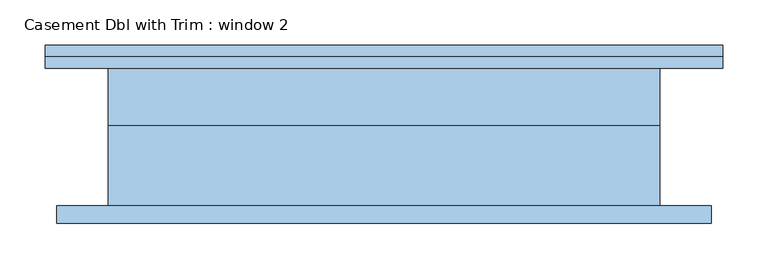
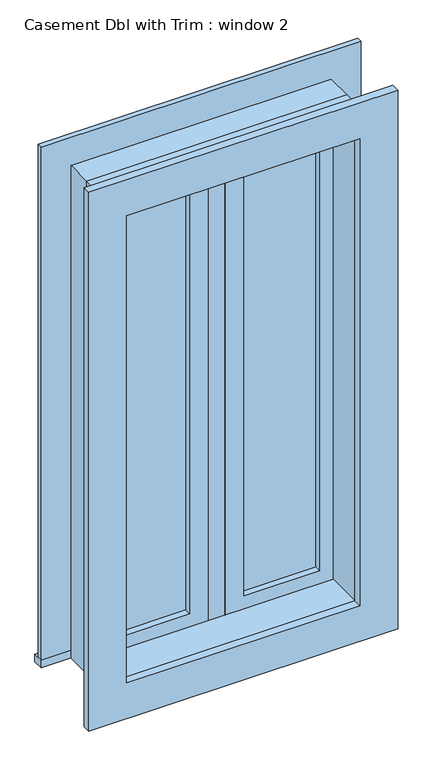
"""IFC4 building model written with IfcOpenShell, lengths in millimetres: window geometry, Casement Dbl with Trim : window 2."""

from ifc_helpers import new_model, si_unit, frame, origin, place, context, project, spatial, polyline, outline, extrude, source, transform, mapped, element, save


def casement_dbl_with_trim_window_2_b083d55d(model_context):
    return source(origin(), model_context, "Body", "SweptSolid", [
        extrude(outline(polyline([(63.5, 60.325), (241.3, 60.325), (241.3, 47.625), (63.5, 47.625), (63.5, 60.325)])), frame((0.0, 0.0, 977.9), z_axis=(0.0, 0.0, 1.0), x_axis=(1.0, 0.0, 0.0)), (0.0, 0.0, 1.0), 1092.2),
        extrude(outline(polyline([(2114.55, 19.05), (933.45, 19.05), (933.45, 285.75), (2114.55, 285.75), (2114.55, 19.05)]), holes=[polyline([(2070.1, 63.5), (2070.1, 241.3), (977.9, 241.3), (977.9, 63.5), (2070.1, 63.5)])]), frame((0.0, 31.75, 0.0), z_axis=(0.0, 1.0, 0.0), x_axis=(0.0, 0.0, 1.0)), (0.0, 0.0, 1.0), 44.45),
        extrude(outline(polyline([(19.05, 31.75), (-19.05, 31.75), (-19.05, 95.25), (19.05, 95.25), (19.05, 31.75)])), frame((0.0, 0.0, 933.45), z_axis=(0.0, 0.0, 1.0), x_axis=(1.0, 0.0, 0.0)), (0.0, 0.0, 1.0), 1181.1),
        extrude(outline(polyline([(-374.65, 120.65), (374.65, 120.65), (374.65, 95.25), (-374.65, 95.25), (-374.65, 120.65)])), frame((0.0, 0.0, 914.4), z_axis=(0.0, 0.0, 1.0), x_axis=(1.0, 0.0, 0.0)), (0.0, 0.0, 1.0), 19.05),
        extrude(outline(polyline([(2114.55, -285.75), (2114.55, 285.75), (933.45, 285.75), (933.45, 374.65), (2203.45, 374.65), (2203.45, -374.65), (933.45, -374.65), (933.45, -285.75), (2114.55, -285.75)])), frame((0.0, 95.25, 0.0), z_axis=(0.0, 1.0, 0.0), x_axis=(0.0, 0.0, 1.0)), (0.0, 0.0, 1.0), 12.7),
        extrude(outline(polyline([(2190.75, 361.95), (2190.75, -361.95), (857.25, -361.95), (857.25, 361.95), (2190.75, 361.95)]), holes=[polyline([(2101.85, 273.05), (946.15, 273.05), (946.15, -273.05), (2101.85, -273.05), (2101.85, 273.05)])]), frame((0.0, -76.2, 0.0), z_axis=(0.0, 1.0, 0.0), x_axis=(0.0, 0.0, 1.0)), (0.0, 0.0, 1.0), 19.05),
        extrude(outline(polyline([(-63.5, 47.625), (-241.3, 47.625), (-241.3, 60.325), (-63.5, 60.325), (-63.5, 47.625)])), frame((0.0, 0.0, 977.9), z_axis=(0.0, 0.0, 1.0), x_axis=(1.0, 0.0, 0.0)), (0.0, 0.0, 1.0), 1092.2),
        extrude(outline(polyline([(2114.55, -285.75), (933.45, -285.75), (933.45, -19.05), (2114.55, -19.05), (2114.55, -285.75)]), holes=[polyline([(2070.1, -241.3), (2070.1, -63.5), (977.9, -63.5), (977.9, -241.3), (2070.1, -241.3)])]), frame((0.0, 31.75, 0.0), z_axis=(0.0, 1.0, 0.0), x_axis=(0.0, 0.0, 1.0)), (0.0, 0.0, 1.0), 44.45),
        extrude(outline(polyline([(2133.6, -304.8), (914.4, -304.8), (914.4, 304.8), (2133.6, 304.8), (2133.6, -304.8)]), holes=[polyline([(2101.85, -273.05), (2101.85, 273.05), (946.15, 273.05), (946.15, -273.05), (2101.85, -273.05)])]), frame((0.0, -57.15, 0.0), z_axis=(0.0, 1.0, 0.0), x_axis=(0.0, 0.0, 1.0)), (0.0, 0.0, 1.0), 88.9),
        extrude(outline(polyline([(2133.6, 304.8), (2133.6, -304.8), (914.4, -304.8), (914.4, 304.8), (2133.6, 304.8)]), holes=[polyline([(2114.55, 285.75), (933.45, 285.75), (933.45, -285.75), (2114.55, -285.75), (2114.55, 285.75)])]), frame((0.0, 31.75, 0.0), z_axis=(0.0, 1.0, 0.0), x_axis=(0.0, 0.0, 1.0)), (0.0, 0.0, 1.0), 63.5),
    ])


if __name__ == "__main__":
    model = new_model("IFC4")
    model_context = context("Model", 3, world=origin())
    ifc_project = project(units=[si_unit("LENGTHUNIT", "METRE", prefix="MILLI")], contexts=[model_context])
    site = spatial("IfcSite", under=ifc_project)
    building = spatial("IfcBuilding", under=site)
    placement = place(None, origin())
    casement_dbl_with_trim_window_2_shape = casement_dbl_with_trim_window_2_b083d55d(model_context)
    element("IfcWindow", 1, ObjectType="Casement Dbl with Trim : window 2", at=placement, inside=building, context=model_context, shape_type="MappedRepresentation", body=[
        mapped(casement_dbl_with_trim_window_2_shape, transform((0.0, 0.0, 0.0), x_axis=(1.0, 0.0, 0.0), y_axis=(0.0, 1.0, 0.0), z_axis=(0.0, 0.0, 1.0))),
    ])
    save(model, "model.ifc")

# Revit data of these elements
# Type "Casement Dbl with Trim : window 2"
#   Type Mark = "13"
#   Construction Type Id = "GSP4R"
#   Assembly Code = "B2020100"
#   Analytic Construction = "1/8 in Pilkington single glazing"
#   Visual Light Transmittance = 0.9
#   Solar Heat Gain Coefficient = 0.78
#   Heat Transfer Coefficient (U) = 0.6496 BTU/(h·ft²·°F)
#   Height = 4' - 0"
#   Default Sill Height = 3' - 0"
#   Trim Projection - Ext. = 0' - 0 1/2"
#   Trim Projection - Int. = 0' - 0 3/4"
#   Trim Width - Exterior = 0' - 3 1/2"
#   Trim Width - Interior = 0' - 3 1/2"
#   Width = 2' - 0"
#   Window Inset = 0' - 0 3/4"
#   Define Thermal Properties by = 1
#   Glass Pane Material = Glass
#   Sash Material = Sash
#   Trim Exterior Material = Trim
#   Trim Interior Material = Trim
#   Wall Closure = (empty or 0)
# Element 1 (IfcWindow, "Casement Dbl with Trim : window 2")
#   Materials on its faces: "Sash", "Trim", "Glass"
# Materials
#   "Glass": class "Glass", colour RGB 0 128 192, transparency 0.75, Description = "Soda Lime Glass", Cost = 0
#   "Sash": class "Wood", colour RGB 224 178 126, transparency 0
#   "Trim": class "Wood", colour RGB 224 178 126, transparency 0
